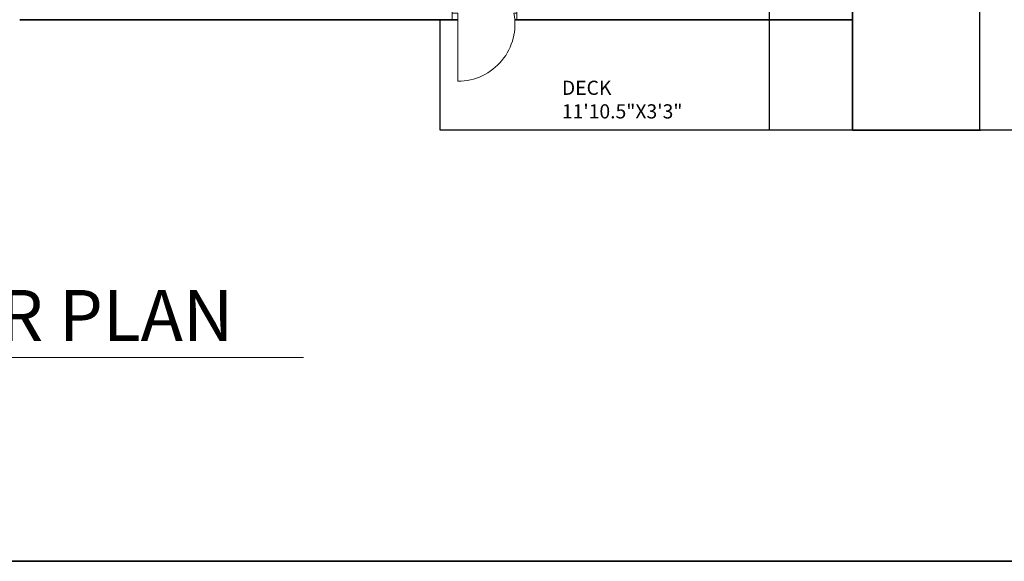
# Model space of a CAD drawing. Units: inches. Extents: x 2120 to 4013, y 1390 to 3019.
# Tile 16 of 59: x 2716 to 3063, y 1390 to 1582. Entities that reach past the tile are written whole.
import ezdxf

# ---------------------------------------------------------------- set-up
doc = ezdxf.new("R2010")
doc.units = ezdxf.units.IN
for name, color, linetype, lineweight in [('A-ANNO-DIMS', 2, 'Continuous', 18), ('A-ANNO-TEXT', 7, 'Continuous', 18), ('A-ANNO-TTLB', 7, 'Continuous', 35), ('A-AREA-IDEN', 7, 'Continuous', 18), ('A-DOOR', 3, 'Continuous', 18), ('A-FLOR-DECK', 7, 'Continuous', 25), ('A-WALL', 7, 'Continuous', 35), ('A-WALL-PATT', 252, 'Continuous', 13)]:
    doc.layers.add(name, color=color, linetype=linetype, lineweight=lineweight)
doc.styles.get("Standard").update_dxf_attribs({"font": 'arial.ttf'})
doc.dimstyles.get("Standard").update_dxf_attribs({"dimtxt": 0.18, "dimasz": 0.18, "dimexe": 0.18, "dimexo": 0.0625, "dimgap": 0.09, "dimtad": 0, "dimtih": 1, "dimtoh": 1, "dimdec": 4, "dimzin": 0, "dimdsep": 46, "dimtxsty": 'Standard', "dimcen": 0.09, "dimadec": 0, "dimazin": 0, "dimtfac": 1, "dimtdec": 4, "dimtofl": 0, "dimtmove": 0, "dimatfit": 3, "dimfxl": 1, "dimtolj": 1, "dimtzin": 0, "dimarcsym": 0})

# ---------------------------------------------------------------- blocks, each defined once
blk = doc.blocks.new('DOOR-SWING-24IN-100p95DEG')
for p, q in [((0, 26.25), (0, 21.75)), ((22.8, 26.25), (22.8, 21.75)), ((0, 21.75), (0, 24)), ((0, 24), (2, 24)), ((2, 24), (2, 0)), ((22.8, 24), (21.8, 24)), ((22.8, 21.75), (22.8, 24))]:
    blk.add_line(p, q)
blk.add_arc((2, 20.17), 20.17, 270, 10.9508)
blk = doc.blocks.new('*D212')
at = {"layer": 'A-ANNO-DIMS', "color": 0, "lineweight": -2, "transparency": 16777216}
for p, q in [((3009.8, 2352.53), (3054.91, 2352.53)), ((3054.73, 2352.35), (3054.73, 1947.71)), ((3054.73, 1542.71), (3054.73, 1947.35)), ((3009.8, 1542.53), (3054.91, 1542.53))]:
    blk.add_line(p, q, dxfattribs=at)
at = {"layer": 'A-ANNO-DIMS', "color": 0, "transparency": 16777216}
for points in [[(3054.7, 2352.35), (3054.76, 2352.35), (3054.73, 2352.53)], [(3054.7, 1542.71), (3054.76, 1542.71), (3054.73, 1542.53)]]:
    blk.add_solid(points, dxfattribs=at)
at = {"layer": 'Defpoints', "color": 0, "transparency": 16777216}
for p in [(3009.73, 2352.53), (3009.73, 1542.53), (3054.73, 1542.53)]:
    blk.add_point(p, dxfattribs=at)
at = {"layer": 'A-ANNO-DIMS', "color": 0, "transparency": 16777216, "insert": (3054.73, 1947.53), "char_height": 0.18, "attachment_point": 5}
blk.add_mtext('\\A1;810', dxfattribs=at)
blk = doc.blocks.new('*D217')
at = {"layer": 'A-ANNO-DIMS', "color": 0, "lineweight": -2, "transparency": 16777216}
for p, q in [((3071.67, 2352.53), (2980.31, 2352.53)), ((2980.49, 2352.35), (2980.49, 1947.71)), ((2980.49, 1542.71), (2980.49, 1947.35)), ((3305.67, 1542.53), (2980.31, 1542.53))]:
    blk.add_line(p, q, dxfattribs=at)
at = {"layer": 'A-ANNO-DIMS', "color": 0, "transparency": 16777216}
for points in [[(2980.46, 2352.35), (2980.52, 2352.35), (2980.49, 2352.53)], [(2980.46, 1542.71), (2980.52, 1542.71), (2980.49, 1542.53)]]:
    blk.add_solid(points, dxfattribs=at)
at = {"layer": 'Defpoints', "color": 0, "transparency": 16777216}
for p in [(2980.49, 2352.53), (3071.73, 2352.53), (3305.73, 1542.53)]:
    blk.add_point(p, dxfattribs=at)
at = {"layer": 'A-ANNO-DIMS', "color": 0, "transparency": 16777216, "insert": (2980.49, 1947.53), "char_height": 0.18, "attachment_point": 5}
blk.add_mtext('\\A1;810', dxfattribs=at)

msp = doc.modelspace()

# ---------------------------------------------------------------- hatches: boundary and pattern name
at = {"layer": 'A-WALL-PATT'}
h = msp.add_hatch(dxfattribs=at)
h.set_pattern_fill('ANSI32', color=256)
h.paths.add_polyline_path([(2271.7331, 2343.531), (2283.3788, 2343.531), (2283.3788, 2348.031), (2283.3788, 2352.5306), (2262.7331, 2352.5306), (2262.7331, 2182.638), (2267.2331, 2182.638), (2271.7331, 2182.638), (2271.7331, 2219.031), (2391.7331, 2219.031), (2391.7331, 2214.189), (2393.9831, 2214.189), (2396.2331, 2214.189), (2396.2331, 2219.031), (2420.2331, 2219.031), (2420.2331, 2225.7535), (2417.2197, 2225.7535), (2415.7331, 2225.7535), (2415.7331, 2223.5306), (2271.7331, 2223.5306)])
h.paths.add_polyline_path([(2380.0942, 2352.5306), (2343.3788, 2352.5306), (2343.3788, 2343.531), (2363.2331, 2343.531), (2363.2331, 2288.8489), (2365.4831, 2288.8489), (2367.7331, 2288.8489), (2367.7331, 2343.531), (2380.0942, 2343.531)], flags=17)
h.paths.add_polyline_path([(2432.4339, 2352.5306), (2404.0943, 2352.5306), (2404.0943, 2343.531), (2415.7331, 2343.531), (2415.7331, 2264.0306), (2367.7331, 2264.0306), (2367.7331, 2266.4872), (2363.2331, 2266.4872), (2363.2331, 2259.531), (2367.7331, 2259.531), (2415.7331, 2259.531), (2415.7331, 2255.0658), (2420.2331, 2255.0658), (2420.2331, 2259.531), (2424.5717, 2259.531), (2424.5717, 2261.781), (2424.5717, 2264.0306), (2420.2331, 2264.0306), (2420.2331, 2343.531), (2432.4339, 2343.531)])
h.paths.add_polyline_path([(2508.9115, 2352.5306), (2456.4339, 2352.5306), (2456.4339, 2343.531), (2468.2331, 2343.531), (2468.2331, 2264.0306), (2448.0487, 2264.0306), (2448.0487, 2259.531), (2468.2331, 2259.531), (2468.2331, 2255.5496), (2472.7331, 2255.5496), (2472.7331, 2343.531), (2508.9115, 2343.531)])
h.paths.add_polyline_path([(2637.7331, 2352.5306), (2544.9116, 2352.5306), (2544.9116, 2343.531), (2589.7331, 2343.531), (2633.2331, 2343.531), (2637.7331, 2343.531)])
h.paths.add_polyline_path([(2594.2331, 2343.5306), (2589.7331, 2343.5306), (2589.7331, 2259.5306), (2589.7331, 2252.4915), (2591.9831, 2252.4915), (2594.2331, 2252.4915)])
h.paths.add_polyline_path([(2637.7331, 2223.5306), (2594.2331, 2223.5306), (2594.2331, 2230.1988), (2591.9831, 2230.1988), (2589.7331, 2230.1988), (2589.7331, 2223.5306), (2472.7331, 2223.5306), (2468.2331, 2223.5306), (2468.2331, 2219.031), (2628.7331, 2219.031), (2628.7331, 2138.031), (2637.7331, 2138.031)])
h.paths.add_polyline_path([(3822.6535, 2458.4402), (3874.9468, 2458.4402), (3874.9468, 2476.9866), (3822.6535, 2476.9866)], flags=9)
h.paths.add_polyline_path([(3834.6921, 2781.8174), (3935.9206, 2781.8174), (3935.9206, 2800.3638), (3834.6921, 2800.3638)], flags=9)
h.paths.add_polyline_path([(3832.2843, 2837.9683), (3884.5776, 2837.9683), (3884.5776, 2856.5146), (3832.2843, 2856.5146)], flags=9)
h.paths.add_polyline_path([(3830.9388, 2861.4782), (3956.8958, 2861.4782), (3956.8958, 2880.0245), (3830.9388, 2880.0245)], flags=9)
h.paths.add_polyline_path([(3870.6966, 2352.5752), (3887.9272, 2352.5752), (3887.9272, 2377.3037), (3870.6966, 2377.3037)], flags=9)
h.paths.add_polyline_path([(3289.2701, 2413.161), (3435.2223, 2413.161), (3435.2223, 2450.2538), (3289.2701, 2450.2538)], flags=9)
h.paths.add_polyline_path([(2487.6944, 2414.3601), (2637.8335, 2414.3601), (2637.8335, 2451.4528), (2487.6944, 2451.4528)], flags=9)
h.paths.add_polyline_path([(2567.3724, 1457.9199), (2815.296, 1457.9199), (2815.296, 1495.0127), (2567.3724, 1495.0127)], flags=9)
h.paths.add_polyline_path([(2655.3825, 2093.2363), (2685.9555, 2093.2363), (2685.9555, 2111.8937), (2655.3825, 2111.8937)], flags=9)
h.paths.add_polyline_path([(2543.9218, 1550.6671), (2587.8406, 1550.6671), (2587.8406, 1569.3244), (2543.9218, 1569.3244)], flags=9)
h.paths.add_polyline_path([(2905.1384, 1543.8113), (2949.0572, 1543.8113), (2949.0572, 1562.4686), (2905.1384, 1562.4686)], flags=9)
h.paths.add_polyline_path([(2736.4118, 1702.4736), (2784.2153, 1702.4736), (2784.2153, 1721.1309), (2736.4118, 1721.1309)], flags=9)
h.paths.add_polyline_path([(2912.8666, 1710.4168), (2951.707, 1710.4168), (2951.707, 1729.0741), (2912.8666, 1729.0741)], flags=9)
h.paths.add_polyline_path([(2923.5785, 1763.5038), (2959.7279, 1763.5038), (2959.7279, 1782.1611), (2923.5785, 1782.1611)], flags=9)
h.paths.add_polyline_path([(2925.2114, 1809.6137), (2967.1861, 1809.6137), (2967.1861, 1828.271), (2925.2114, 1828.271)], flags=9)
h.paths.add_polyline_path([(2996.2711, 1878.9003), (2996.2711, 1913.109), (2977.6138, 1913.109), (2977.6138, 1878.9003)], flags=9)
h.paths.add_polyline_path([(2883.0859, 1895.7192), (2927.1855, 1895.7192), (2927.1855, 1914.3766), (2883.0859, 1914.3766)], flags=9)
h.paths.add_polyline_path([(2787.3924, 1810.8013), (2841.0213, 1810.8013), (2841.0213, 1829.4587), (2787.3924, 1829.4587)], flags=9)
h.paths.add_polyline_path([(2775.6399, 2101.7395), (2829.2689, 2101.7395), (2829.2689, 2120.3968), (2775.6399, 2120.3968)], flags=9)
h.paths.add_polyline_path([(2913.0263, 2075.817), (2951.8667, 2075.817), (2951.8667, 2094.4744), (2913.0263, 2094.4744)], flags=9)
h.paths.add_polyline_path([(2929.966, 2133.3669), (2966.1154, 2133.3669), (2966.1154, 2152.0243), (2929.966, 2152.0243)], flags=9)
h.paths.add_polyline_path([(2932.7502, 2182.6088), (2968.8996, 2182.6088), (2968.8996, 2201.2662), (2932.7502, 2201.2662)], flags=9)
h.paths.add_polyline_path([(2996.0681, 2266.3173), (2996.0681, 2300.5261), (2977.4108, 2300.5261), (2977.4108, 2266.3173)], flags=9)
h.paths.add_polyline_path([(2885.1039, 2279.2186), (2929.2035, 2279.2186), (2929.2035, 2297.8759), (2885.1039, 2297.8759)], flags=9)
h.paths.add_polyline_path([(2735.7042, 2218.3197), (2783.5078, 2218.3197), (2783.5078, 2236.9771), (2735.7042, 2236.9771)], flags=9)
h.paths.add_polyline_path([(2635.6049, 2044.0085), (2648.9678, 2044.0085), (2648.9678, 2054.312), (2635.6049, 2054.312)], flags=9)
h.paths.add_polyline_path([(2714.0148, 1923.0473), (2727.3777, 1923.0473), (2727.3777, 1933.3508), (2714.0148, 1933.3508)], flags=9)
h.paths.add_polyline_path([(2709.0345, 1988.1628), (2722.3974, 1988.1628), (2722.3974, 1998.4663), (2709.0345, 1998.4663)], flags=9)
h.paths.add_polyline_path([(2592.8935, 1962.1763), (2606.2564, 1962.1763), (2606.2564, 1972.4799), (2592.8935, 1972.4799)], flags=9)
h.paths.add_polyline_path([(2618.3996, 1985.9724), (2644.1942, 1985.9724), (2644.1942, 1996.2759), (2618.3996, 1996.2759)], flags=9)
h.paths.add_polyline_path([(2601.279, 1920.5869), (2614.6419, 1920.5869), (2614.6419, 1930.8904), (2601.279, 1930.8904)], flags=9)
h.paths.add_polyline_path([(2692.3278, 1932.7645), (2704.5311, 1932.7645), (2704.5311, 1943.0681), (2692.3278, 1943.0681)], flags=9)
h.paths.add_polyline_path([(2311.122, 1672.7318), (2355.0408, 1672.7318), (2355.0408, 1691.3892), (2311.122, 1691.3892)], flags=9)
h.paths.add_polyline_path([(2456.2551, 1632.3198), (2492.4796, 1632.3198), (2492.4796, 1650.9772), (2456.2551, 1650.9772)], flags=9)
h.paths.add_polyline_path([(2401.0766, 1631.4793), (2437.301, 1631.4793), (2437.301, 1650.1367), (2401.0766, 1650.1367)], flags=9)
h.paths.add_polyline_path([(2546.7054, 1700.9235), (2594.509, 1700.9235), (2594.509, 1719.5809), (2546.7054, 1719.5809)], flags=9)
h.paths.add_polyline_path([(2445.4866, 1766.9937), (2497.5261, 1766.9937), (2497.5261, 1785.651), (2445.4866, 1785.651)], flags=9)
h.paths.add_polyline_path([(2287.9992, 1739.7675), (2326.8396, 1739.7675), (2326.8396, 1758.4248), (2287.9992, 1758.4248)], flags=9)
h.paths.add_polyline_path([(2458.5279, 1924.7607), (2510.5675, 1924.7607), (2510.5675, 1943.4181), (2458.5279, 1943.4181)], flags=9)
h.paths.add_polyline_path([(2309.2811, 1902.7642), (2345.4305, 1902.7642), (2345.4305, 1921.4215), (2309.2811, 1921.4215)], flags=9)
h.paths.add_polyline_path([(2490.7554, 2018.9392), (2530.7896, 2018.9392), (2530.7896, 2037.5965), (2490.7554, 2037.5965)], flags=9)
h.paths.add_polyline_path([(2402.143, 2024.7393), (2438.5414, 2024.7393), (2438.5414, 2043.3966), (2402.143, 2043.3966)], flags=9)
h.paths.add_polyline_path([(2287.856, 1931.7926), (2326.6964, 1931.7926), (2326.6964, 1950.4499), (2287.856, 1950.4499)], flags=9)
h.paths.add_polyline_path([(2281.7979, 2193.5771), (2320.6383, 2193.5771), (2320.6383, 2212.2344), (2281.7979, 2212.2344)], flags=25)
h.paths.add_polyline_path([(2484.0754, 2093.892), (2536.115, 2093.892), (2536.115, 2112.5494), (2484.0754, 2112.5494)], flags=9)
h.paths.add_polyline_path([(2624.7948, 2281.8639), (2624.7948, 2311.4137), (2606.1375, 2311.4137), (2606.1375, 2281.8639)], flags=9)
h.paths.add_polyline_path([(2507.5036, 2290.3639), (2541.934, 2290.3639), (2541.934, 2309.0212), (2507.5036, 2309.0212)], flags=9)
h.paths.add_polyline_path([(2423.1076, 2285.2202), (2459.332, 2285.2202), (2459.332, 2303.8776), (2423.1076, 2303.8776)], flags=9)
h.paths.add_polyline_path([(2374.5467, 2289.6272), (2410.7711, 2289.6272), (2410.7711, 2308.2846), (2374.5467, 2308.2846)], flags=25)
h.paths.add_polyline_path([(2277.4907, 2227.5651), (2316.3311, 2227.5651), (2316.3311, 2246.2224), (2277.4907, 2246.2224)], flags=25)
h.paths.add_polyline_path([(2655.3825, 2093.2367), (2685.9555, 2093.2367), (2685.9555, 2111.894), (2655.3825, 2111.894)], flags=9)
h.paths.add_polyline_path([(2543.9217, 1550.6674), (2587.8406, 1550.6674), (2587.8406, 1569.3247), (2543.9217, 1569.3247)], flags=9)
h.paths.add_polyline_path([(2905.1384, 1543.8116), (2949.0572, 1543.8116), (2949.0572, 1562.4689), (2905.1384, 1562.4689)], flags=9)
h.paths.add_polyline_path([(2736.4118, 1702.4739), (2784.2153, 1702.4739), (2784.2153, 1721.1312), (2736.4118, 1721.1312)], flags=9)
h.paths.add_polyline_path([(2912.8666, 1710.4171), (2951.707, 1710.4171), (2951.707, 1729.0744), (2912.8666, 1729.0744)], flags=9)
h.paths.add_polyline_path([(2923.5785, 1763.5041), (2959.7279, 1763.5041), (2959.7279, 1782.1614), (2923.5785, 1782.1614)], flags=9)
h.paths.add_polyline_path([(2925.2114, 1809.614), (2967.1861, 1809.614), (2967.1861, 1828.2713), (2925.2114, 1828.2713)], flags=9)
h.paths.add_polyline_path([(2996.2711, 1878.9006), (2996.2711, 1913.1094), (2977.6137, 1913.1094), (2977.6137, 1878.9006)], flags=9)
h.paths.add_polyline_path([(2883.0859, 1895.7195), (2927.1855, 1895.7195), (2927.1855, 1914.3769), (2883.0859, 1914.3769)], flags=9)
h.paths.add_polyline_path([(2787.3924, 1810.8016), (2841.0213, 1810.8016), (2841.0213, 1829.459), (2787.3924, 1829.459)], flags=9)
h.paths.add_polyline_path([(2775.6399, 2101.7398), (2829.2688, 2101.7398), (2829.2688, 2120.3971), (2775.6399, 2120.3971)], flags=9)
h.paths.add_polyline_path([(2913.0263, 2075.8173), (2951.8667, 2075.8173), (2951.8667, 2094.4747), (2913.0263, 2094.4747)], flags=9)
h.paths.add_polyline_path([(2929.966, 2133.3672), (2966.1154, 2133.3672), (2966.1154, 2152.0246), (2929.966, 2152.0246)], flags=9)
h.paths.add_polyline_path([(2932.7502, 2182.6091), (2968.8996, 2182.6091), (2968.8996, 2201.2665), (2932.7502, 2201.2665)], flags=9)
h.paths.add_polyline_path([(2996.0681, 2266.3176), (2996.0681, 2300.5264), (2977.4108, 2300.5264), (2977.4108, 2266.3176)], flags=9)
h.paths.add_polyline_path([(2885.1039, 2279.2189), (2929.2035, 2279.2189), (2929.2035, 2297.8762), (2885.1039, 2297.8762)], flags=9)
h.paths.add_polyline_path([(2735.7042, 2218.32), (2783.5078, 2218.32), (2783.5078, 2236.9774), (2735.7042, 2236.9774)], flags=9)
h.paths.add_polyline_path([(2635.6048, 2044.0088), (2648.9677, 2044.0088), (2648.9677, 2054.3123), (2635.6048, 2054.3123)], flags=9)
h.paths.add_polyline_path([(2714.0148, 1923.0476), (2727.3777, 1923.0476), (2727.3777, 1933.3511), (2714.0148, 1933.3511)], flags=9)
h.paths.add_polyline_path([(2709.0345, 1988.1631), (2722.3974, 1988.1631), (2722.3974, 1998.4666), (2709.0345, 1998.4666)], flags=9)
h.paths.add_polyline_path([(2592.8935, 1962.1766), (2606.2564, 1962.1766), (2606.2564, 1972.4802), (2592.8935, 1972.4802)], flags=9)
h.paths.add_polyline_path([(2618.3995, 1985.9727), (2644.1942, 1985.9727), (2644.1942, 1996.2762), (2618.3995, 1996.2762)], flags=9)
h.paths.add_polyline_path([(2601.279, 1920.5872), (2614.6419, 1920.5872), (2614.6419, 1930.8908), (2601.279, 1930.8908)], flags=9)
h.paths.add_polyline_path([(2692.3278, 1932.7648), (2704.5311, 1932.7648), (2704.5311, 1943.0684), (2692.3278, 1943.0684)], flags=9)
h.paths.add_polyline_path([(2311.122, 1672.7321), (2355.0408, 1672.7321), (2355.0408, 1691.3895), (2311.122, 1691.3895)], flags=9)
h.paths.add_polyline_path([(2456.2551, 1632.3201), (2492.4795, 1632.3201), (2492.4795, 1650.9775), (2456.2551, 1650.9775)], flags=9)
h.paths.add_polyline_path([(2401.0766, 1631.4796), (2437.301, 1631.4796), (2437.301, 1650.137), (2401.0766, 1650.137)], flags=9)
h.paths.add_polyline_path([(2546.7054, 1700.9238), (2594.509, 1700.9238), (2594.509, 1719.5812), (2546.7054, 1719.5812)], flags=9)
h.paths.add_polyline_path([(2445.4866, 1766.994), (2497.5261, 1766.994), (2497.5261, 1785.6513), (2445.4866, 1785.6513)], flags=9)
h.paths.add_polyline_path([(2287.9992, 1739.7678), (2326.8396, 1739.7678), (2326.8396, 1758.4251), (2287.9992, 1758.4251)], flags=9)
h.paths.add_polyline_path([(2458.5279, 1924.7611), (2510.5675, 1924.7611), (2510.5675, 1943.4184), (2458.5279, 1943.4184)], flags=9)
h.paths.add_polyline_path([(2309.2811, 1902.7645), (2345.4305, 1902.7645), (2345.4305, 1921.4218), (2309.2811, 1921.4218)], flags=9)
h.paths.add_polyline_path([(2490.7554, 2018.9395), (2530.7895, 2018.9395), (2530.7895, 2037.5968), (2490.7554, 2037.5968)], flags=9)
h.paths.add_polyline_path([(2402.143, 2024.7396), (2438.5413, 2024.7396), (2438.5413, 2043.3969), (2402.143, 2043.3969)], flags=9)
h.paths.add_polyline_path([(2287.856, 1931.7929), (2326.6964, 1931.7929), (2326.6964, 1950.4502), (2287.856, 1950.4502)], flags=9)
h.paths.add_polyline_path([(2281.7979, 2193.5774), (2320.6383, 2193.5774), (2320.6383, 2212.2347), (2281.7979, 2212.2347)], flags=25)
h.paths.add_polyline_path([(2484.0754, 2093.8924), (2536.115, 2093.8924), (2536.115, 2112.5497), (2484.0754, 2112.5497)], flags=9)
h.paths.add_polyline_path([(2624.7948, 2281.8642), (2624.7948, 2311.414), (2606.1374, 2311.414), (2606.1374, 2281.8642)], flags=9)
h.paths.add_polyline_path([(2507.5035, 2290.3642), (2541.934, 2290.3642), (2541.934, 2309.0215), (2507.5035, 2309.0215)], flags=9)
h.paths.add_polyline_path([(2423.1075, 2285.2205), (2459.332, 2285.2205), (2459.332, 2303.8779), (2423.1075, 2303.8779)], flags=9)
h.paths.add_polyline_path([(2374.5467, 2289.6275), (2410.7711, 2289.6275), (2410.7711, 2308.2849), (2374.5467, 2308.2849)], flags=25)
h.paths.add_polyline_path([(2277.4907, 2227.5654), (2316.3311, 2227.5654), (2316.3311, 2246.2227), (2277.4907, 2246.2227)], flags=25)
h = msp.add_hatch(dxfattribs=at)
h.set_pattern_fill('ANSI32', color=256)
h.paths.add_polyline_path([(2271.7331, 1980.389), (2262.7331, 1980.389), (2262.7331, 1912.8434), (2267.2331, 1912.8434), (2271.7331, 1912.8434), (2271.7331, 1922.531), (2351.2331, 1922.531), (2351.2331, 1901.4728), (2355.7331, 1901.4728), (2355.7331, 1922.531), (2357.9815, 1922.531), (2357.9815, 1926.5306), (2271.7331, 1926.5306)])
h.paths.add_polyline_path([(2589.2331, 1949.1622), (2584.7331, 1949.1622), (2580.2331, 1949.1622), (2580.2331, 1874.5306), (2355.7331, 1874.5306), (2355.7331, 1880.1922), (2351.2331, 1880.1922), (2351.2331, 1874.5306), (2271.7331, 1874.5306), (2271.7331, 1888.8431), (2262.7331, 1888.8431), (2262.7331, 1842.2909), (2267.2331, 1842.2909), (2271.7331, 1842.2909), (2271.7331, 1865.531), (2415.7331, 1865.531), (2415.7331, 1779.7286), (2420.2331, 1779.7286), (2420.2331, 1865.531), (2589.2331, 1865.531)])
h.paths.add_polyline_path([(2271.7331, 1782.2906), (2262.7331, 1782.2906), (2262.7331, 1711.4639), (2267.2331, 1711.4639), (2271.7331, 1711.4639), (2271.7331, 1738.031), (2420.2331, 1738.031), (2420.2331, 1742.531), (2420.2331, 1747.3376), (2417.9831, 1747.3376), (2415.7331, 1747.3376), (2415.7331, 1742.5306), (2271.7331, 1742.5306)])
h.paths.add_polyline_path([(2271.7331, 1627.031), (2362.3957, 1627.031), (2362.3957, 1629.281), (2362.3957, 1631.5306), (2271.7331, 1631.5306), (2271.7331, 1675.4636), (2262.7331, 1675.4636), (2262.7331, 1581.531), (2405.3032, 1581.531), (2405.3032, 1586.031), (2405.3032, 1590.5306), (2396.2331, 1590.5306), (2396.2331, 1691.4513), (2418.7206, 1691.4513), (2418.7206, 1695.951), (2396.2331, 1695.951), (2391.7331, 1695.951), (2391.7331, 1631.5306), (2386.7425, 1631.5306), (2386.7425, 1629.2806), (2386.7425, 1627.031), (2391.7331, 1627.031), (2391.7331, 1586.1709), (2271.7331, 1586.1709)])
h.paths.add_polyline_path([(2459.6703, 1590.5306), (2429.3032, 1590.5306), (2429.3032, 1581.531), (2459.6703, 1581.531), (2459.6703, 1586.031)])
h.paths.add_polyline_path([(2501.2331, 1590.531), (2501.2331, 1665.0195), (2498.9831, 1665.0195), (2496.7331, 1665.0195), (2496.7331, 1590.5306), (2483.8201, 1590.5306), (2483.8201, 1590.1579), (2483.6704, 1590.1579), (2483.6704, 1581.531), (2505.0196, 1581.531), (2505.0196, 1583.781), (2505.0196, 1586.0306), (2501.2331, 1586.0306)])
h.paths.add_polyline_path([(2544.1361, 1583.781), (2544.1361, 1586.0306), (2527.1368, 1586.0306), (2527.1368, 1583.7806), (2527.1368, 1581.531), (2544.1361, 1581.531)])
h.paths.add_polyline_path([(3822.6535, 2458.4402), (3874.9468, 2458.4402), (3874.9468, 2476.9866), (3822.6535, 2476.9866)], flags=9)
h.paths.add_polyline_path([(3834.6921, 2781.8174), (3935.9206, 2781.8174), (3935.9206, 2800.3638), (3834.6921, 2800.3638)], flags=9)
h.paths.add_polyline_path([(3832.2843, 2837.9683), (3884.5776, 2837.9683), (3884.5776, 2856.5146), (3832.2843, 2856.5146)], flags=9)
h.paths.add_polyline_path([(3830.9388, 2861.4782), (3956.8958, 2861.4782), (3956.8958, 2880.0245), (3830.9388, 2880.0245)], flags=9)
h.paths.add_polyline_path([(3870.6966, 2352.5752), (3887.9272, 2352.5752), (3887.9272, 2377.3037), (3870.6966, 2377.3037)], flags=9)
h.paths.add_polyline_path([(3289.2701, 2413.161), (3435.2223, 2413.161), (3435.2223, 2450.2538), (3289.2701, 2450.2538)], flags=9)
h.paths.add_polyline_path([(2487.6944, 2414.3601), (2637.8335, 2414.3601), (2637.8335, 2451.4528), (2487.6944, 2451.4528)], flags=9)
h.paths.add_polyline_path([(2567.3724, 1457.9199), (2815.296, 1457.9199), (2815.296, 1495.0127), (2567.3724, 1495.0127)], flags=9)
h.paths.add_polyline_path([(2655.3825, 2093.2363), (2685.9555, 2093.2363), (2685.9555, 2111.8937), (2655.3825, 2111.8937)], flags=9)
h.paths.add_polyline_path([(2543.9218, 1550.6671), (2587.8406, 1550.6671), (2587.8406, 1569.3244), (2543.9218, 1569.3244)], flags=9)
h.paths.add_polyline_path([(2905.1384, 1543.8113), (2949.0572, 1543.8113), (2949.0572, 1562.4686), (2905.1384, 1562.4686)], flags=9)
h.paths.add_polyline_path([(2736.4118, 1702.4736), (2784.2153, 1702.4736), (2784.2153, 1721.1309), (2736.4118, 1721.1309)], flags=9)
h.paths.add_polyline_path([(2912.8666, 1710.4168), (2951.707, 1710.4168), (2951.707, 1729.0741), (2912.8666, 1729.0741)], flags=9)
h.paths.add_polyline_path([(2923.5785, 1763.5038), (2959.7279, 1763.5038), (2959.7279, 1782.1611), (2923.5785, 1782.1611)], flags=9)
h.paths.add_polyline_path([(2925.2114, 1809.6137), (2967.1861, 1809.6137), (2967.1861, 1828.271), (2925.2114, 1828.271)], flags=9)
h.paths.add_polyline_path([(2996.2711, 1878.9003), (2996.2711, 1913.109), (2977.6138, 1913.109), (2977.6138, 1878.9003)], flags=9)
h.paths.add_polyline_path([(2883.0859, 1895.7192), (2927.1855, 1895.7192), (2927.1855, 1914.3766), (2883.0859, 1914.3766)], flags=9)
h.paths.add_polyline_path([(2787.3924, 1810.8013), (2841.0213, 1810.8013), (2841.0213, 1829.4587), (2787.3924, 1829.4587)], flags=9)
h.paths.add_polyline_path([(2775.6399, 2101.7395), (2829.2689, 2101.7395), (2829.2689, 2120.3968), (2775.6399, 2120.3968)], flags=9)
h.paths.add_polyline_path([(2913.0263, 2075.817), (2951.8667, 2075.817), (2951.8667, 2094.4744), (2913.0263, 2094.4744)], flags=9)
h.paths.add_polyline_path([(2929.966, 2133.3669), (2966.1154, 2133.3669), (2966.1154, 2152.0243), (2929.966, 2152.0243)], flags=9)
h.paths.add_polyline_path([(2932.7502, 2182.6088), (2968.8996, 2182.6088), (2968.8996, 2201.2662), (2932.7502, 2201.2662)], flags=9)
h.paths.add_polyline_path([(2996.0681, 2266.3173), (2996.0681, 2300.5261), (2977.4108, 2300.5261), (2977.4108, 2266.3173)], flags=9)
h.paths.add_polyline_path([(2885.1039, 2279.2186), (2929.2035, 2279.2186), (2929.2035, 2297.8759), (2885.1039, 2297.8759)], flags=9)
h.paths.add_polyline_path([(2735.7042, 2218.3197), (2783.5078, 2218.3197), (2783.5078, 2236.9771), (2735.7042, 2236.9771)], flags=9)
h.paths.add_polyline_path([(2635.6049, 2044.0085), (2648.9678, 2044.0085), (2648.9678, 2054.312), (2635.6049, 2054.312)], flags=9)
h.paths.add_polyline_path([(2714.0148, 1923.0473), (2727.3777, 1923.0473), (2727.3777, 1933.3508), (2714.0148, 1933.3508)], flags=9)
h.paths.add_polyline_path([(2709.0345, 1988.1628), (2722.3974, 1988.1628), (2722.3974, 1998.4663), (2709.0345, 1998.4663)], flags=9)
h.paths.add_polyline_path([(2592.8935, 1962.1763), (2606.2564, 1962.1763), (2606.2564, 1972.4799), (2592.8935, 1972.4799)], flags=9)
h.paths.add_polyline_path([(2618.3996, 1985.9724), (2644.1942, 1985.9724), (2644.1942, 1996.2759), (2618.3996, 1996.2759)], flags=9)
h.paths.add_polyline_path([(2601.279, 1920.5869), (2614.6419, 1920.5869), (2614.6419, 1930.8904), (2601.279, 1930.8904)], flags=9)
h.paths.add_polyline_path([(2692.3278, 1932.7645), (2704.5311, 1932.7645), (2704.5311, 1943.0681), (2692.3278, 1943.0681)], flags=9)
h.paths.add_polyline_path([(2311.122, 1672.7318), (2355.0408, 1672.7318), (2355.0408, 1691.3892), (2311.122, 1691.3892)], flags=25)
h.paths.add_polyline_path([(2456.2551, 1632.3198), (2492.4796, 1632.3198), (2492.4796, 1650.9772), (2456.2551, 1650.9772)], flags=9)
h.paths.add_polyline_path([(2401.0766, 1631.4793), (2437.301, 1631.4793), (2437.301, 1650.1367), (2401.0766, 1650.1367)], flags=9)
h.paths.add_polyline_path([(2546.7054, 1700.9235), (2594.509, 1700.9235), (2594.509, 1719.5809), (2546.7054, 1719.5809)], flags=9)
h.paths.add_polyline_path([(2445.4866, 1766.9937), (2497.5261, 1766.9937), (2497.5261, 1785.651), (2445.4866, 1785.651)], flags=9)
h.paths.add_polyline_path([(2287.9992, 1739.7675), (2326.8396, 1739.7675), (2326.8396, 1758.4248), (2287.9992, 1758.4248)], flags=24)
h.paths.add_polyline_path([(2458.5279, 1924.7607), (2510.5675, 1924.7607), (2510.5675, 1943.4181), (2458.5279, 1943.4181)], flags=25)
h.paths.add_polyline_path([(2309.2811, 1902.7642), (2345.4305, 1902.7642), (2345.4305, 1921.4215), (2309.2811, 1921.4215)], flags=25)
h.paths.add_polyline_path([(2490.7554, 2018.9392), (2530.7896, 2018.9392), (2530.7896, 2037.5965), (2490.7554, 2037.5965)], flags=9)
h.paths.add_polyline_path([(2402.143, 2024.7393), (2438.5414, 2024.7393), (2438.5414, 2043.3966), (2402.143, 2043.3966)], flags=9)
h.paths.add_polyline_path([(2287.856, 1931.7926), (2326.6964, 1931.7926), (2326.6964, 1950.4499), (2287.856, 1950.4499)], flags=25)
h.paths.add_polyline_path([(2281.7979, 2193.5771), (2320.6383, 2193.5771), (2320.6383, 2212.2344), (2281.7979, 2212.2344)], flags=9)
h.paths.add_polyline_path([(2484.0754, 2093.892), (2536.115, 2093.892), (2536.115, 2112.5494), (2484.0754, 2112.5494)], flags=9)
h.paths.add_polyline_path([(2624.7948, 2281.8639), (2624.7948, 2311.4137), (2606.1375, 2311.4137), (2606.1375, 2281.8639)], flags=9)
h.paths.add_polyline_path([(2507.5036, 2290.3639), (2541.934, 2290.3639), (2541.934, 2309.0212), (2507.5036, 2309.0212)], flags=9)
h.paths.add_polyline_path([(2423.1076, 2285.2202), (2459.332, 2285.2202), (2459.332, 2303.8776), (2423.1076, 2303.8776)], flags=9)
h.paths.add_polyline_path([(2374.5467, 2289.6272), (2410.7711, 2289.6272), (2410.7711, 2308.2846), (2374.5467, 2308.2846)], flags=9)
h.paths.add_polyline_path([(2277.4907, 2227.5651), (2316.3311, 2227.5651), (2316.3311, 2246.2224), (2277.4907, 2246.2224)], flags=9)
h.paths.add_polyline_path([(2655.3825, 2093.2367), (2685.9555, 2093.2367), (2685.9555, 2111.894), (2655.3825, 2111.894)], flags=9)
h.paths.add_polyline_path([(2543.9217, 1550.6674), (2587.8406, 1550.6674), (2587.8406, 1569.3247), (2543.9217, 1569.3247)], flags=9)
h.paths.add_polyline_path([(2905.1384, 1543.8116), (2949.0572, 1543.8116), (2949.0572, 1562.4689), (2905.1384, 1562.4689)], flags=9)
h.paths.add_polyline_path([(2736.4118, 1702.4739), (2784.2153, 1702.4739), (2784.2153, 1721.1312), (2736.4118, 1721.1312)], flags=9)
h.paths.add_polyline_path([(2912.8666, 1710.4171), (2951.707, 1710.4171), (2951.707, 1729.0744), (2912.8666, 1729.0744)], flags=9)
h.paths.add_polyline_path([(2923.5785, 1763.5041), (2959.7279, 1763.5041), (2959.7279, 1782.1614), (2923.5785, 1782.1614)], flags=9)
h.paths.add_polyline_path([(2925.2114, 1809.614), (2967.1861, 1809.614), (2967.1861, 1828.2713), (2925.2114, 1828.2713)], flags=9)
h.paths.add_polyline_path([(2996.2711, 1878.9006), (2996.2711, 1913.1094), (2977.6137, 1913.1094), (2977.6137, 1878.9006)], flags=9)
h.paths.add_polyline_path([(2883.0859, 1895.7195), (2927.1855, 1895.7195), (2927.1855, 1914.3769), (2883.0859, 1914.3769)], flags=9)
h.paths.add_polyline_path([(2787.3924, 1810.8016), (2841.0213, 1810.8016), (2841.0213, 1829.459), (2787.3924, 1829.459)], flags=9)
h.paths.add_polyline_path([(2775.6399, 2101.7398), (2829.2688, 2101.7398), (2829.2688, 2120.3971), (2775.6399, 2120.3971)], flags=9)
h.paths.add_polyline_path([(2913.0263, 2075.8173), (2951.8667, 2075.8173), (2951.8667, 2094.4747), (2913.0263, 2094.4747)], flags=9)
h.paths.add_polyline_path([(2929.966, 2133.3672), (2966.1154, 2133.3672), (2966.1154, 2152.0246), (2929.966, 2152.0246)], flags=9)
h.paths.add_polyline_path([(2932.7502, 2182.6091), (2968.8996, 2182.6091), (2968.8996, 2201.2665), (2932.7502, 2201.2665)], flags=9)
h.paths.add_polyline_path([(2996.0681, 2266.3176), (2996.0681, 2300.5264), (2977.4108, 2300.5264), (2977.4108, 2266.3176)], flags=9)
h.paths.add_polyline_path([(2885.1039, 2279.2189), (2929.2035, 2279.2189), (2929.2035, 2297.8762), (2885.1039, 2297.8762)], flags=9)
h.paths.add_polyline_path([(2735.7042, 2218.32), (2783.5078, 2218.32), (2783.5078, 2236.9774), (2735.7042, 2236.9774)], flags=9)
h.paths.add_polyline_path([(2635.6048, 2044.0088), (2648.9677, 2044.0088), (2648.9677, 2054.3123), (2635.6048, 2054.3123)], flags=9)
h.paths.add_polyline_path([(2714.0148, 1923.0476), (2727.3777, 1923.0476), (2727.3777, 1933.3511), (2714.0148, 1933.3511)], flags=9)
h.paths.add_polyline_path([(2709.0345, 1988.1631), (2722.3974, 1988.1631), (2722.3974, 1998.4666), (2709.0345, 1998.4666)], flags=9)
h.paths.add_polyline_path([(2592.8935, 1962.1766), (2606.2564, 1962.1766), (2606.2564, 1972.4802), (2592.8935, 1972.4802)], flags=9)
h.paths.add_polyline_path([(2618.3995, 1985.9727), (2644.1942, 1985.9727), (2644.1942, 1996.2762), (2618.3995, 1996.2762)], flags=9)
h.paths.add_polyline_path([(2601.279, 1920.5872), (2614.6419, 1920.5872), (2614.6419, 1930.8908), (2601.279, 1930.8908)], flags=9)
h.paths.add_polyline_path([(2692.3278, 1932.7648), (2704.5311, 1932.7648), (2704.5311, 1943.0684), (2692.3278, 1943.0684)], flags=9)
h.paths.add_polyline_path([(2311.122, 1672.7321), (2355.0408, 1672.7321), (2355.0408, 1691.3895), (2311.122, 1691.3895)], flags=25)
h.paths.add_polyline_path([(2456.2551, 1632.3201), (2492.4795, 1632.3201), (2492.4795, 1650.9775), (2456.2551, 1650.9775)], flags=9)
h.paths.add_polyline_path([(2401.0766, 1631.4796), (2437.301, 1631.4796), (2437.301, 1650.137), (2401.0766, 1650.137)], flags=9)
h.paths.add_polyline_path([(2546.7054, 1700.9238), (2594.509, 1700.9238), (2594.509, 1719.5812), (2546.7054, 1719.5812)], flags=9)
h.paths.add_polyline_path([(2445.4866, 1766.994), (2497.5261, 1766.994), (2497.5261, 1785.6513), (2445.4866, 1785.6513)], flags=9)
h.paths.add_polyline_path([(2287.9992, 1739.7678), (2326.8396, 1739.7678), (2326.8396, 1758.4251), (2287.9992, 1758.4251)], flags=24)
h.paths.add_polyline_path([(2458.5279, 1924.7611), (2510.5675, 1924.7611), (2510.5675, 1943.4184), (2458.5279, 1943.4184)], flags=25)
h.paths.add_polyline_path([(2309.2811, 1902.7645), (2345.4305, 1902.7645), (2345.4305, 1921.4218), (2309.2811, 1921.4218)], flags=25)
h.paths.add_polyline_path([(2490.7554, 2018.9395), (2530.7895, 2018.9395), (2530.7895, 2037.5968), (2490.7554, 2037.5968)], flags=9)
h.paths.add_polyline_path([(2402.143, 2024.7396), (2438.5413, 2024.7396), (2438.5413, 2043.3969), (2402.143, 2043.3969)], flags=9)
h.paths.add_polyline_path([(2287.856, 1931.7929), (2326.6964, 1931.7929), (2326.6964, 1950.4502), (2287.856, 1950.4502)], flags=25)
h.paths.add_polyline_path([(2281.7979, 2193.5774), (2320.6383, 2193.5774), (2320.6383, 2212.2347), (2281.7979, 2212.2347)], flags=9)
h.paths.add_polyline_path([(2484.0754, 2093.8924), (2536.115, 2093.8924), (2536.115, 2112.5497), (2484.0754, 2112.5497)], flags=9)
h.paths.add_polyline_path([(2624.7948, 2281.8642), (2624.7948, 2311.414), (2606.1374, 2311.414), (2606.1374, 2281.8642)], flags=9)
h.paths.add_polyline_path([(2507.5035, 2290.3642), (2541.934, 2290.3642), (2541.934, 2309.0215), (2507.5035, 2309.0215)], flags=9)
h.paths.add_polyline_path([(2423.1075, 2285.2205), (2459.332, 2285.2205), (2459.332, 2303.8779), (2423.1075, 2303.8779)], flags=9)
h.paths.add_polyline_path([(2374.5467, 2289.6275), (2410.7711, 2289.6275), (2410.7711, 2308.2849), (2374.5467, 2308.2849)], flags=9)
h.paths.add_polyline_path([(2277.4907, 2227.5654), (2316.3311, 2227.5654), (2316.3311, 2246.2227), (2277.4907, 2246.2227)], flags=9)

# ---------------------------------------------------------------- linework, layer by layer
at = {"layer": 'A-ANNO-TEXT'}
msp.add_line((2815.8947, 1462.19), (2566.6873, 1462.19), dxfattribs=at)
at = {"layer": 'A-ANNO-TTLB'}
msp.add_lwpolyline([(2120.4581, 3019.1237), (4012.9334, 3019.1237), (4012.9334, 1390.2222), (2120.4581, 1390.2222)], close=True, dxfattribs=at)
at = {"layer": 'A-FLOR-DECK'}
for p, q in [((2864.2331, 1542.531), (2864.2331, 1581.531)), ((2864.2331, 1542.5306), (2864.2331, 1581.5306)), ((3009.7331, 1542.531), (2864.2331, 1542.531)), ((3009.7331, 1542.5306), (2864.2331, 1542.5306))]:
    msp.add_line(p, q, dxfattribs=at)
at = {"layer": 'A-WALL'}
for p, q in [((3009.7331, 1962.531), (3009.7331, 1542.531)), ((3009.7331, 1962.5306), (3009.7331, 1542.5306)), ((2870.4124, 1581.5306), (2715.7331, 1581.5306)), ((3009.7331, 1581.5306), (2890.5189, 1581.5306))]:
    msp.add_line(p, q, dxfattribs=at)

# ---------------------------------------------------------------- block references
at = {"layer": 'A-DOOR'}
for p in [(2868.4123, 1559.781), (2868.4124, 1559.7806)]:
    msp.add_blockref('DOOR-SWING-24IN-100p95DEG', p, dxfattribs=at)

# ---------------------------------------------------------------- texts
at = {"layer": 'A-ANNO-TEXT', "insert": (2573.9352, 1486.0679), "char_height": 18, "attachment_point": 1}
msp.add_mtext_dynamic_manual_height_columns('FIRST FLOOR PLAN', width=524.266688, gutter_width=12.5, heights=[0], dxfattribs=at)
at = {"layer": 'A-AREA-IDEN', "char_height": 5, "attachment_point": 1}
for insert in [(2907.1489, 1559.9808), (2907.149, 1559.9805)]:
    msp.add_mtext_dynamic_manual_height_columns('DECK\\P11\'10.5"X3\'3"', width=168.800767, gutter_width=12.5, heights=[0], dxfattribs=dict(at, insert=insert))

# ---------------------------------------------------------------- dimensions: what is measured, and where the dimension line sits
at = {"layer": 'A-ANNO-DIMS'}
for base, p1, p2, picture, middle in [((2980.4877, 2352.531), (3305.7347, 1542.531), (3071.7347, 2352.531), '*D217', (2980.4877, 1947.531)), ((3054.7331, 1542.531), (3009.7331, 2352.531), (3009.7331, 1542.531), '*D212', (3054.7331, 1947.531))]:
    dim = msp.add_linear_dim(base=base, p1=p1, p2=p2, angle=90, dimstyle='Standard', override={"dimdec": 0, "dimlfac": 1, "dimrnd": 0, "dimzin": 0, "dimdsep": 46, "dimlunit": 2}, dxfattribs=at)
    dim.commit()
    dim.dimension.update_dxf_attribs({"geometry": picture, "text_midpoint": middle})

doc.saveas('drawing.dxf')
